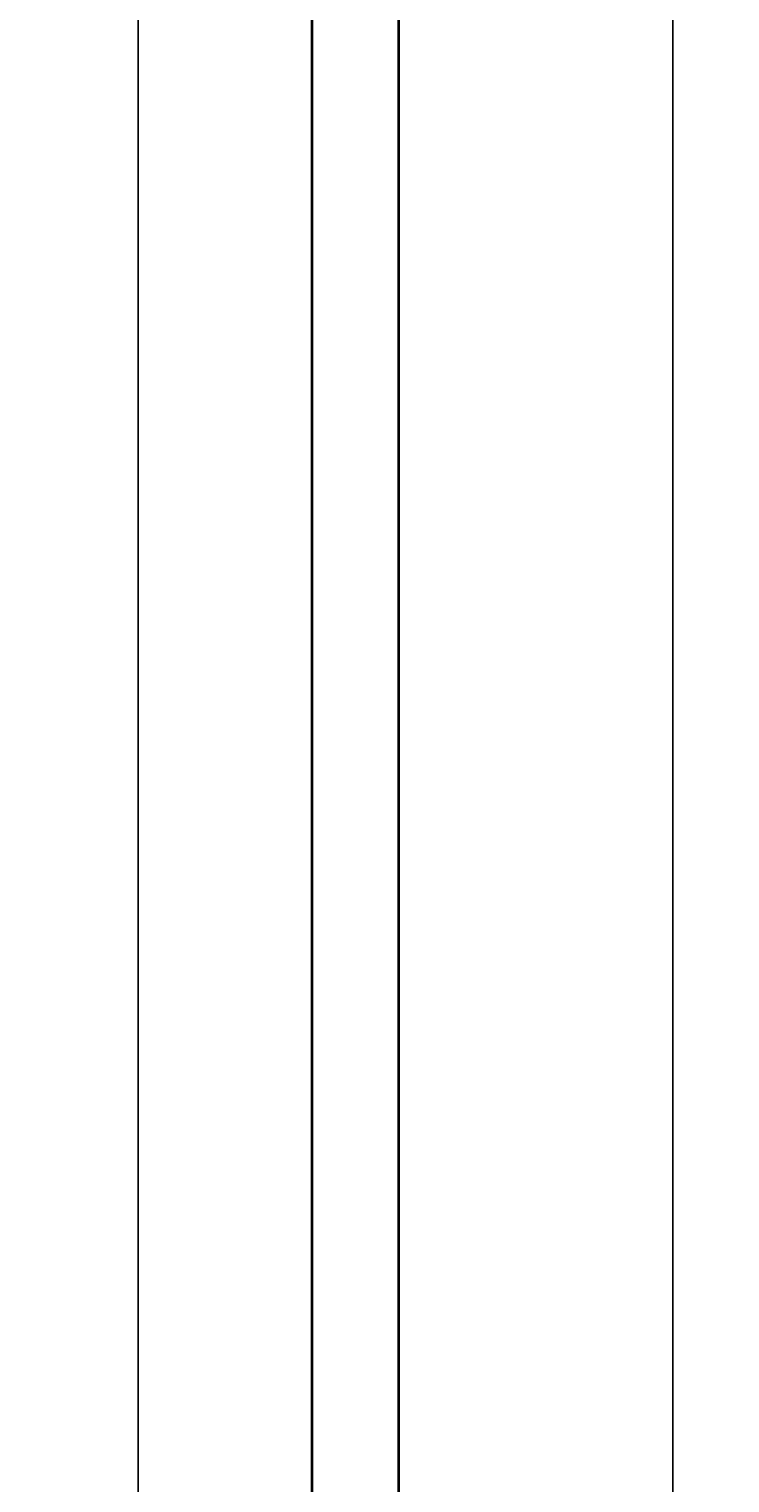
# Model space of a CAD drawing. Units: inches. Extents: x -10 to 502, y -868 to 56.
# Tile 2 of 14: x 6 to 78, y -724 to -573. Entities that reach past the tile are written whole.
import ezdxf

# ---------------------------------------------------------------- set-up
doc = ezdxf.new("R2010")
doc.units = ezdxf.units.IN
doc.header["$MEASUREMENT"] = 0
for name, color, linetype, lineweight in [('A-ANNO-DIMS', 2, 'Continuous', 18), ('A-WALL', 7, 'Continuous', 35), ('L-WALL', 7, 'Continuous', 35)]:
    doc.layers.add(name, color=color, linetype=linetype, lineweight=lineweight)
doc.styles.get("Standard").update_dxf_attribs({"font": 'arial.ttf'})
doc.dimstyles.get("Standard").update_dxf_attribs({"dimtxt": 0.18, "dimasz": 0.18, "dimexe": 0.18, "dimexo": 0.0625, "dimgap": 0.09, "dimtad": 0, "dimtih": 1, "dimtoh": 1, "dimdec": 0, "dimzin": 0, "dimdsep": 46, "dimlunit": 3, "dimtxsty": 'Standard', "dimcen": 0.09, "dimadec": 0, "dimazin": 0, "dimtfac": 1, "dimtdec": 0, "dimtofl": 0, "dimtmove": 0, "dimatfit": 3, "dimfxl": 1, "dimtolj": 1, "dimtzin": 0, "dimarcsym": 0})

# ---------------------------------------------------------------- blocks, each defined once
blk = doc.blocks.new('*D2')
at = {"layer": 'A-ANNO-DIMS', "color": 0, "lineweight": -2, "transparency": 16777216}
for p, q in [((34.89, 12.15), (16.75, 12.15)), ((16.93, 11.97), (16.93, -376.2)), ((16.93, -770.67), (16.93, -382.51)), ((34.89, -770.85), (16.75, -770.85))]:
    blk.add_line(p, q, dxfattribs=at)
at = {"layer": 'A-ANNO-DIMS', "color": 0, "transparency": 16777216}
for points in [[(16.9, 11.97), (16.96, 11.97), (16.93, 12.15)], [(16.9, -770.67), (16.96, -770.67), (16.93, -770.85)]]:
    blk.add_solid(points, dxfattribs=at)
at = {"layer": 'Defpoints', "color": 0, "transparency": 16777216}
for p in [(34.95, 12.15), (16.93, -770.85), (34.95, -770.85)]:
    blk.add_point(p, dxfattribs=at)
at = {"layer": 'A-ANNO-DIMS', "color": 0, "transparency": 16777216, "insert": (16.93, -379.35), "char_height": 6, "attachment_point": 5}
blk.add_mtext('\\A1;65\'-3"', dxfattribs=at)
blk = doc.blocks.new('*D48')
at = {"layer": 'A-ANNO-DIMS', "color": 0, "lineweight": -2, "transparency": 16777216}
for p, q in [((43.95, -332.92), (43.95, -846.58)), ((72.45, -332.92), (72.45, -846.58)), ((44.13, -846.4), (57.66, -846.4)), ((72.27, -846.4), (58.74, -846.4))]:
    blk.add_line(p, q, dxfattribs=at)
at = {"layer": 'A-ANNO-DIMS', "color": 0, "transparency": 16777216}
for points in [[(44.13, -846.37), (44.13, -846.43), (43.95, -846.4)], [(72.27, -846.37), (72.27, -846.43), (72.45, -846.4)]]:
    blk.add_solid(points, dxfattribs=at)
at = {"layer": 'Defpoints', "color": 0, "transparency": 16777216}
for p in [(43.95, -332.85), (72.45, -332.85), (72.45, -846.4)]:
    blk.add_point(p, dxfattribs=at)
at = {"layer": 'A-ANNO-DIMS', "color": 0, "transparency": 16777216, "insert": (58.2, -846.4), "char_height": 0.18, "attachment_point": 5}
blk.add_mtext('\\A1;2\'-4 1/2"', dxfattribs=at)
blk = doc.blocks.new('*D56')
at = {"layer": 'A-ANNO-DIMS', "color": 0, "lineweight": -2, "transparency": 16777216}
for p, q in [((43.95, -549.92), (43.95, -846.58)), ((93.07, -549.92), (93.07, -846.58)), ((44.13, -846.4), (68.18, -846.4)), ((92.89, -846.4), (68.84, -846.4))]:
    blk.add_line(p, q, dxfattribs=at)
at = {"layer": 'A-ANNO-DIMS', "color": 0, "transparency": 16777216}
for points in [[(44.13, -846.37), (44.13, -846.43), (43.95, -846.4)], [(92.89, -846.37), (92.89, -846.43), (93.07, -846.4)]]:
    blk.add_solid(points, dxfattribs=at)
at = {"layer": 'Defpoints', "color": 0, "transparency": 16777216}
for p in [(43.95, -549.85), (93.07, -549.85), (43.95, -846.4)]:
    blk.add_point(p, dxfattribs=at)
at = {"layer": 'A-ANNO-DIMS', "color": 0, "transparency": 16777216, "insert": (68.51, -846.4), "char_height": 0.18, "attachment_point": 5}
blk.add_mtext('\\A1;4\'-1"', dxfattribs=at)

msp = doc.modelspace()

# ---------------------------------------------------------------- linework, layer by layer
at = {"layer": 'A-WALL'}
msp.add_line((34.95, 12.15), (34.95, -770.85), dxfattribs=at)
at = {"layer": 'L-WALL'}
msp.add_line((43.95, -549.85), (43.95, -770.85), dxfattribs=at)

# ---------------------------------------------------------------- dimensions: what is measured, and where the dimension line sits
at = {"layer": 'A-ANNO-DIMS'}
dim = msp.add_linear_dim(base=(16.93, -770.85), p1=(34.95, 12.15), p2=(34.95, -770.85), angle=90, dimstyle='Standard', override={"dimtxt": 6, "dimclrd": 0, "dimclre": 0, "dimclrt": 0}, dxfattribs=at)
dim.commit()
dim.dimension.update_dxf_attribs({"geometry": '*D2', "text_midpoint": (16.93, -379.35)})
for base, p1, p2, picture, middle in [((72.45, -846.4), (43.95, -332.85), (72.45, -332.85), '*D48', (58.2, -846.4)), ((43.95, -846.4), (93.07, -549.85), (43.95, -549.85), '*D56', (68.51, -846.4))]:
    dim = msp.add_linear_dim(base=base, p1=p1, p2=p2, dimstyle='Standard', override={"dimdec": 1, "dimlfac": 1, "dimrnd": 0, "dimzin": 1, "dimdsep": 46, "dimlunit": 4, "dimfrac": 2}, dxfattribs=at)
    dim.commit()
    dim.dimension.update_dxf_attribs({"geometry": picture, "text_midpoint": middle})

doc.saveas('drawing.dxf')
